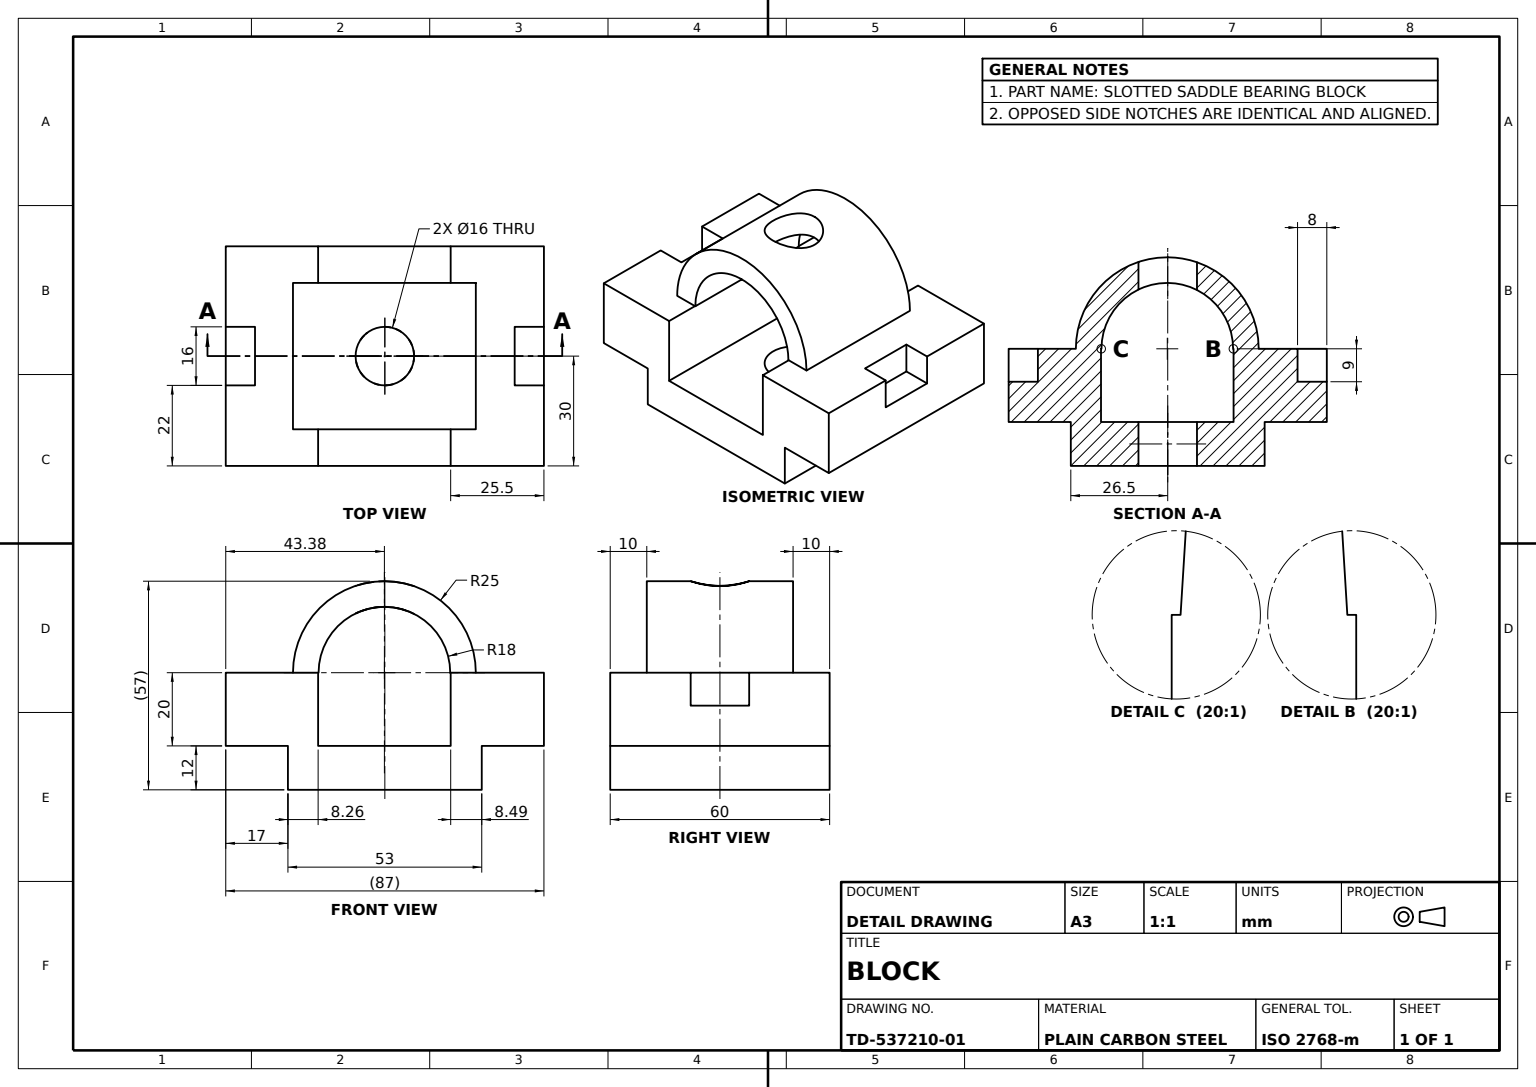
from build123d import *

# Parameters (mm, degrees)
BASE_BLOCK_DEPTH             = 60
SADDLE_ARCH_DEPTH            = 60
BEARING_SEAT_CUT_FRONT_DEPTH = 10
BEARING_START                = -10
BEARING_SEAT_CUT_REAR_DEPTH  = 10
OIL_HOLE_SKETCH_R            = 8
OIL_HOLE_8_DEPTH             = 100
LOCATING_SLOTS_SKETCH_W      = 8
LOCATING_SLOTS_SKETCH_H      = 16
LOCATING_SLOTS_DEPTH         = 9


with BuildPart() as part:
    # Base Block Profile → Base Block (new body)
    with BuildSketch(Plane.XY):
        Polygon((0, 0), (53, 0), (53, 12), (70, 12), (70, 32), (44.5, 32), (44.508364197, 12), (8.257120322, 12), (8.257120322, 32), (-17, 32), (-17, 12), (0, 12), align=None)
    extrude(amount=-BASE_BLOCK_DEPTH)

    # Saddle Arch Profile → Saddle Arch (add)
    with BuildSketch(Plane.XY):
        with BuildLine():
            Line((1.378560161, 32), (8.257120322, 32))
            Line((8.257120322, 32), (8.378560161, 32))
            ThreePointArc((8.378560161, 32), (26.378560161, 50), (44.378560161, 32))
            Line((44.378560161, 32), (44.5, 32))
            Line((44.5, 32), (51.378560161, 32))
            ThreePointArc((51.378560161, 32), (26.378560161, 57), (1.378560161, 32))
        make_face()
    extrude(amount=-SADDLE_ARCH_DEPTH)

    # Bearing Seat Front Profile → Bearing Seat Cut Front (cut)
    with BuildSketch(Plane.XY):
        with BuildLine():
            Line((1.378560161, 32), (8.257120322, 32))
            Line((8.257120322, 32), (8.378560161, 32))
            ThreePointArc((8.378560161, 32), (26.378560161, 50), (44.378560161, 32))
            Line((44.378560161, 32), (44.5, 32))
            Line((44.5, 32), (51.378560161, 32))
            ThreePointArc((51.378560161, 32), (26.378560161, 57), (1.378560161, 32))
        make_face()
    extrude(amount=-BEARING_SEAT_CUT_FRONT_DEPTH, mode=Mode.SUBTRACT)

    # Bearing Seat Rear Profile → Bearing Seat Cut Rear (cut)
    with BuildSketch(Plane(origin=(0, 0, -60), x_dir=(-1, 0, 0), z_dir=(0, 0, -1)).offset(BEARING_START)):
        with BuildLine():
            Line((-51.378560161, 32), (-44.378560161, 32))
            ThreePointArc((-44.378560161, 32), (-26.378560161, 50), (-8.378560161, 32))
            Line((-8.378560161, 32), (-1.378560161, 32))
            ThreePointArc((-1.378560161, 32), (-26.378560161, 57), (-51.378560161, 32))
        make_face()
    extrude(amount=BEARING_SEAT_CUT_REAR_DEPTH, mode=Mode.SUBTRACT)

    # Oil Hole Sketch → Oil Hole Ø8 (cut)
    with BuildSketch(Plane.XZ):
        with Locations(Location((26.5, -30, 0), (0, 0, 270))):
            Circle(OIL_HOLE_SKETCH_R)
    extrude(amount=-OIL_HOLE_8_DEPTH, mode=Mode.SUBTRACT)

    # Locating Slots Sketch → Locating Slots (cut)
    with BuildSketch(Plane(origin=(0, 32, 0), x_dir=(1, 0, 0), z_dir=(0, 1, 0))):
        with Locations((-13, 30)):
            Rectangle(LOCATING_SLOTS_SKETCH_W, LOCATING_SLOTS_SKETCH_H)
        Polygon((70, 30), (70, 38), (62, 38), (62, 22), (70, 22), align=None)
    extrude(amount=-LOCATING_SLOTS_DEPTH, mode=Mode.SUBTRACT)


solid = part.part
